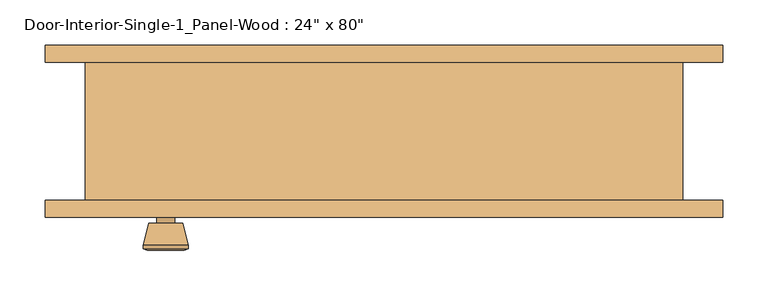
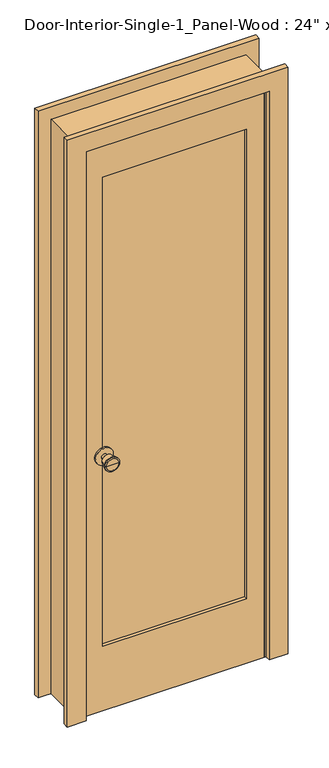
"""IFC4 building model written with IfcOpenShell, lengths in millimetres: door geometry."""

from ifc_helpers import new_model, si_unit, point, frame, frame_2d, origin, place, context, project, spatial, polyline, circle_curve, trimmed, segment, composite_curve, outline, extrude, faceted_brep, source, transform, mapped, element, save
from ifc_brep_helpers import plane_surface, cylinder_surface, revolved_surface, advanced_brep


def door_1d623f84(model_context):
    return source(origin(), model_context, "Body", "SolidModel", [
        advanced_brep(
        [(-241.3, -32.1, 914.4), (-251.3, -32.1, 914.4), (-231.3, -32.1, 914.4), (-220.8241324, 16.9, 914.4), (-261.7758676, 16.9, 914.4), (-241.3, 16.9, 914.4), (-216.3, 15.0721319, 914.4), (-266.3, 15.0721319, 914.4), (-216.3, 11.6084537, 914.4), (-266.3, 11.6084537, 914.4), (-222.663764, -13.1, 914.4), (-259.936236, -13.1, 914.4), (-231.3, -13.1, 914.4), (-251.3, -13.1, 914.4)],
        [
            (0, 1),
            (1, 2, circle_curve(frame((-241.3, -32.1, 914.4), z_axis=(0.0, -1.0, 0.0), x_axis=(-1.0, 0.0, 0.0)), 10.0)),
            (2, 0),
            (2, 1, circle_curve(frame((-241.3, -32.1, 914.4), z_axis=(0.0, -1.0, 0.0), x_axis=(-1.0, 0.0, 0.0)), 10.0)),
            (3, 4, circle_curve(frame((-241.3, 16.9, 914.4), z_axis=(0.0, 1.0, 0.0), x_axis=(-1.0, 0.0, 0.0)), 20.4758676)),
            (4, 5),
            (5, 3),
            (4, 3, circle_curve(frame((-241.3, 16.9, 914.4), z_axis=(0.0, 1.0, 0.0), x_axis=(-1.0, 0.0, 0.0)), 20.4758676)),
            (6, 7, circle_curve(frame((-241.3, 15.0721319, 914.4), z_axis=(0.0, 1.0, 0.0), x_axis=(-1.0, 0.0, 0.0)), 25.0)),
            (7, 4),
            (3, 6),
            (7, 6, circle_curve(frame((-241.3, 15.0721319, 914.4), z_axis=(0.0, 1.0, 0.0), x_axis=(-1.0, 0.0, 0.0)), 25.0)),
            (8, 9, circle_curve(frame((-241.3, 11.6084537, 914.4), z_axis=(0.0, 1.0, 0.0), x_axis=(-1.0, 0.0, 0.0)), 25.0)),
            (9, 7),
            (6, 8),
            (9, 8, circle_curve(frame((-241.3, 11.6084537, 914.4), z_axis=(0.0, 1.0, 0.0), x_axis=(-1.0, 0.0, 0.0)), 25.0)),
            (10, 11, circle_curve(frame((-241.3, -13.1, 914.4), z_axis=(0.0, 1.0, 0.0), x_axis=(-1.0, 0.0, 0.0)), 18.636236)),
            (11, 9),
            (8, 10),
            (11, 10, circle_curve(frame((-241.3, -13.1, 914.4), z_axis=(0.0, 1.0, 0.0), x_axis=(-1.0, 0.0, 0.0)), 18.636236)),
            (12, 13, circle_curve(frame((-241.3, -13.1, 914.4), z_axis=(0.0, 1.0, 0.0), x_axis=(-1.0, 0.0, 0.0)), 10.0)),
            (13, 11),
            (10, 12),
            (13, 12, circle_curve(frame((-241.3, -13.1, 914.4), z_axis=(0.0, 1.0, 0.0), x_axis=(-1.0, 0.0, 0.0)), 10.0)),
            (1, 13),
            (12, 2),
        ],
        [
            plane_surface(frame((-241.3, -32.1, 914.4), z_axis=(0.0, -1.0, 0.0), x_axis=(-1.0, 0.0, 0.0))),
            plane_surface(frame((-241.3, 16.9, 914.4), z_axis=(0.0, 1.0, 0.0), x_axis=(-1.0, 0.0, 0.0))),
            revolved_surface(polyline([(-261.7758676, 16.9, 914.4), (-266.3, 15.0721319, 914.4)]), (-241.3, -32.1, 914.4), (0.0, -1.0, 0.0)),
            cylinder_surface(frame((-241.3, -32.1, 914.4), z_axis=(0.0, -1.0, 0.0), x_axis=(-1.0, 0.0, 0.0)), 25.0),
            revolved_surface(polyline([(-266.3, 11.6084537, 914.4), (-259.936236, -13.1, 914.4)]), (-241.3, -32.1, 914.4), (0.0, -1.0, 0.0)),
            plane_surface(frame((-241.3, -13.1, 914.4), z_axis=(0.0, -1.0, 0.0), x_axis=(-1.0, 0.0, 0.0))),
            cylinder_surface(frame((-241.3, -32.1, 914.4), z_axis=(0.0, -1.0, 0.0), x_axis=(-1.0, 0.0, 0.0)), 10.0),
        ],
        [
            (0, [[1, 2, 3]]),
            (0, [[-3, 4, -1]]),
            (1, [[5, 6, 7]]),
            (1, [[8, -7, -6]]),
            (2, [[9, 10, -5, 11]]),
            (2, [[12, -11, -8, -10]]),
            (3, [[13, 14, -9, 15]]),
            (3, [[16, -15, -12, -14]]),
            (4, [[17, 18, -13, 19]]),
            (4, [[20, -19, -16, -18]]),
            (5, [[21, 22, -17, 23]]),
            (5, [[24, -23, -20, -22]]),
            (6, [[-2, 25, -21, 26]]),
            (6, [[-4, -26, -24, -25]]),
        ],
    ),
        extrude(outline(composite_curve([segment(trimmed(circle_curve(frame_2d((914.4, -241.3)), 30.0), [point((914.4, -271.3))], [point((914.4, -211.3))], False, "CARTESIAN"), True, "CONTINUOUS"), segment(trimmed(circle_curve(frame_2d((914.4, -241.3)), 30.0), [point((914.4, -211.3))], [point((914.4, -271.3))], False, "CARTESIAN"), True, "CONTINUOUS")], self_intersect=False)), frame((0.0, -38.1, 0.0), z_axis=(0.0, 1.0, 0.0), x_axis=(0.0, 0.0, 1.0)), (0.0, 0.0, 1.0), 6.0),
        advanced_brep(
        [(-241.3, -79.025, 914.4), (-231.3, -79.025, 914.4), (-251.3, -79.025, 914.4), (-220.8241324, -128.025, 914.4), (-241.3, -128.025, 914.4), (-261.7758676, -128.025, 914.4), (-216.3, -126.1971319, 914.4), (-266.3, -126.1971319, 914.4), (-216.3, -122.7334537, 914.4), (-266.3, -122.7334537, 914.4), (-222.663764, -98.025, 914.4), (-259.936236, -98.025, 914.4), (-231.3, -98.025, 914.4), (-251.3, -98.025, 914.4)],
        [
            (0, 1),
            (1, 2, circle_curve(frame((-241.3, -79.025, 914.4), z_axis=(0.0, 1.0, 0.0), x_axis=(-1.0, 0.0, 0.0)), 10.0)),
            (2, 0),
            (2, 1, circle_curve(frame((-241.3, -79.025, 914.4), z_axis=(0.0, 1.0, 0.0), x_axis=(-1.0, 0.0, 0.0)), 10.0)),
            (3, 4),
            (4, 5),
            (5, 3, circle_curve(frame((-241.3, -128.025, 914.4), z_axis=(0.0, -1.0, 0.0), x_axis=(-1.0, 0.0, 0.0)), 20.4758676)),
            (3, 5, circle_curve(frame((-241.3, -128.025, 914.4), z_axis=(0.0, -1.0, 0.0), x_axis=(-1.0, 0.0, 0.0)), 20.4758676)),
            (6, 3),
            (5, 7),
            (7, 6, circle_curve(frame((-241.3, -126.1971319, 914.4), z_axis=(0.0, -1.0, 0.0), x_axis=(-1.0, 0.0, 0.0)), 25.0)),
            (6, 7, circle_curve(frame((-241.3, -126.1971319, 914.4), z_axis=(0.0, -1.0, 0.0), x_axis=(-1.0, 0.0, 0.0)), 25.0)),
            (8, 6),
            (7, 9),
            (9, 8, circle_curve(frame((-241.3, -122.7334537, 914.4), z_axis=(0.0, -1.0, 0.0), x_axis=(-1.0, 0.0, 0.0)), 25.0)),
            (8, 9, circle_curve(frame((-241.3, -122.7334537, 914.4), z_axis=(0.0, -1.0, 0.0), x_axis=(-1.0, 0.0, 0.0)), 25.0)),
            (10, 8),
            (9, 11),
            (11, 10, circle_curve(frame((-241.3, -98.025, 914.4), z_axis=(0.0, -1.0, 0.0), x_axis=(-1.0, 0.0, 0.0)), 18.636236)),
            (10, 11, circle_curve(frame((-241.3, -98.025, 914.4), z_axis=(0.0, -1.0, 0.0), x_axis=(-1.0, 0.0, 0.0)), 18.636236)),
            (12, 10),
            (11, 13),
            (13, 12, circle_curve(frame((-241.3, -98.025, 914.4), z_axis=(0.0, -1.0, 0.0), x_axis=(-1.0, 0.0, 0.0)), 10.0)),
            (12, 13, circle_curve(frame((-241.3, -98.025, 914.4), z_axis=(0.0, -1.0, 0.0), x_axis=(-1.0, 0.0, 0.0)), 10.0)),
            (1, 12),
            (13, 2),
        ],
        [
            plane_surface(frame((-241.3, -79.025, 914.4), z_axis=(0.0, 1.0, 0.0), x_axis=(-1.0, 0.0, 0.0))),
            plane_surface(frame((-241.3, -128.025, 914.4), z_axis=(0.0, -1.0, 0.0), x_axis=(-1.0, 0.0, 0.0))),
            revolved_surface(polyline([(-261.7758676, -128.025, 914.4), (-266.3, -126.1971319, 914.4)]), (-241.3, -79.025, 914.4), (0.0, 1.0, 0.0)),
            cylinder_surface(frame((-241.3, -79.025, 914.4), z_axis=(0.0, 1.0, 0.0), x_axis=(-1.0, 0.0, 0.0)), 25.0),
            revolved_surface(polyline([(-266.3, -122.7334537, 914.4), (-259.936236, -98.025, 914.4)]), (-241.3, -79.025, 914.4), (0.0, 1.0, 0.0)),
            plane_surface(frame((-241.3, -98.025, 914.4), z_axis=(0.0, 1.0, 0.0), x_axis=(-1.0, 0.0, 0.0))),
            cylinder_surface(frame((-241.3, -79.025, 914.4), z_axis=(0.0, 1.0, 0.0), x_axis=(-1.0, 0.0, 0.0)), 10.0),
        ],
        [
            (0, [[1, 2, 3]]),
            (0, [[-3, 4, -1]]),
            (1, [[5, 6, 7]]),
            (1, [[-6, -5, 8]]),
            (2, [[9, -7, 10, 11]]),
            (2, [[-10, -8, -9, 12]]),
            (3, [[13, -11, 14, 15]]),
            (3, [[-14, -12, -13, 16]]),
            (4, [[17, -15, 18, 19]]),
            (4, [[-18, -16, -17, 20]]),
            (5, [[21, -19, 22, 23]]),
            (5, [[-22, -20, -21, 24]]),
            (6, [[25, -23, 26, -2]]),
            (6, [[-26, -24, -25, -4]]),
        ],
    ),
        extrude(outline(composite_curve([segment(trimmed(circle_curve(frame_2d((914.4, -241.3)), 30.0), [point((914.4, -271.3))], [point((914.4, -211.3))], False, "CARTESIAN"), True, "CONTINUOUS"), segment(trimmed(circle_curve(frame_2d((914.4, -241.3)), 30.0), [point((914.4, -211.3))], [point((914.4, -271.3))], False, "CARTESIAN"), True, "CONTINUOUS")], self_intersect=False)), frame((0.0, -79.025, 0.0), z_axis=(0.0, 1.0, 0.0), x_axis=(0.0, 0.0, 1.0)), (0.0, 0.0, 1.0), 6.0),
        extrude(outline(polyline([(244.475, -49.7416667), (244.475, -61.3833333), (-244.475, -61.3833333), (-244.475, -49.7416667), (244.475, -49.7416667)])), frame((0.0, 0.0, 231.775), z_axis=(0.0, 0.0, 1.0), x_axis=(1.0, 0.0, 0.0)), (0.0, 0.0, 1.0), 1681.1625),
        extrude(outline(polyline([(2032.0, -304.8), (0.0, -304.8), (0.0, 304.8), (2032.0, 304.8), (2032.0, -304.8)]), holes=[polyline([(1912.9375, -244.475), (1912.9375, 244.475), (231.775, 244.475), (231.775, -244.475), (1912.9375, -244.475)])]), frame((0.0, -73.025, 0.0), z_axis=(0.0, 1.0, 0.0), x_axis=(0.0, 0.0, 1.0)), (0.0, 0.0, 1.0), 34.925),
        faceted_brep([(330.2, -73.025, 0.0), (304.8, -73.025, 0.0), (304.8, -38.1, 0.0), (292.1, -38.1, 0.0), (292.1, -3.175, 0.0), (304.8, -3.175, 0.0), (304.8, 79.375, 0.0), (330.2, 79.375, 0.0), (330.2, 79.375, 2057.4), (330.2, -73.025, 2057.4), (304.8, 79.375, 2032.0), (-304.8, 79.375, 2032.0), (-304.8, 79.375, 0.0), (-330.2, 79.375, 0.0), (-330.2, 79.375, 2057.4), (304.8, -3.175, 2032.0), (292.1, -3.175, 2019.3), (-292.1, -3.175, 2019.3), (-292.1, -3.175, 0.0), (-304.8, -3.175, 0.0), (-304.8, -3.175, 2032.0), (292.1, -38.1, 2019.3), (304.8, -38.1, 2032.0), (-304.8, -38.1, 2032.0), (-304.8, -38.1, 0.0), (-292.1, -38.1, 0.0), (-292.1, -38.1, 2019.3), (304.8, -73.025, 2032.0), (-330.2, -73.025, 2057.4), (-330.2, -73.025, 0.0), (-304.8, -73.025, 0.0), (-304.8, -73.025, 2032.0)], [[[0, 1, 2, 3, 4, 5, 6, 7]], [[7, 8, 9, 0]], [[6, 10, 11, 12, 13, 14, 8, 7]], [[5, 15, 10, 6]], [[4, 16, 17, 18, 19, 20, 15, 5]], [[3, 21, 16, 4]], [[2, 22, 23, 24, 25, 26, 21, 3]], [[1, 27, 22, 2]], [[0, 9, 28, 29, 30, 31, 27, 1]], [[8, 14, 28, 9]], [[15, 20, 11, 10]], [[21, 26, 17, 16]], [[27, 31, 23, 22]], [[29, 13, 12, 19, 18, 25, 24, 30]], [[14, 13, 29, 28]], [[20, 19, 12, 11]], [[26, 25, 18, 17]], [[31, 30, 24, 23]]]),
        extrude(outline(polyline([(0.0, 374.65), (2101.85, 374.65), (2101.85, -374.65), (0.0, -374.65), (0.0, -311.15), (2038.35, -311.15), (2038.35, 311.15), (0.0, 311.15), (0.0, 374.65)])), frame((0.0, 79.375, 0.0), z_axis=(0.0, 1.0, 0.0), x_axis=(0.0, 0.0, 1.0)), (0.0, 0.0, 1.0), 19.05),
        extrude(outline(polyline([(0.0, 374.65), (2101.85, 374.65), (2101.85, -374.65), (0.0, -374.65), (0.0, -311.15), (2038.35, -311.15), (2038.35, 311.15), (0.0, 311.15), (0.0, 374.65)])), frame((0.0, -92.075, 0.0), z_axis=(0.0, 1.0, 0.0), x_axis=(0.0, 0.0, 1.0)), (0.0, 0.0, 1.0), 19.05),
    ])


if __name__ == "__main__":
    model = new_model("IFC4")
    model_context = context("Model", 3, world=origin())
    ifc_project = project(units=[si_unit("LENGTHUNIT", "METRE", prefix="MILLI")], contexts=[model_context])
    site = spatial("IfcSite", under=ifc_project)
    building = spatial("IfcBuilding", under=site)
    placement = place(None, origin())
    door_shape = door_1d623f84(model_context)
    element("IfcDoor", 1, ObjectType="Door-Interior-Single-1_Panel-Wood : 24\" x 80\"", at=placement, inside=building, context=model_context, shape_type="MappedRepresentation", body=[
        mapped(door_shape, transform((0.0, 0.0, 0.0), x_axis=(1.0, 0.0, 0.0), y_axis=(0.0, 1.0, 0.0), z_axis=(0.0, 0.0, 1.0))),
    ])
    save(model, "model.ifc")

# Revit data of these elements
# Type "Door-Interior-Single-1_Panel-Wood : 24\" x 80\""
#   Type Mark = "12"
#   Assembly Code = "C1020300"
#   Analytic Construction = "Wooden"
#   Top Rail = 0' - 4 11/16"
#   Thickness = 0' - 1 3/8"
#   Thermal Resistance (R) = 2.5876 (h·ft²·°F)/BTU
#   Swing Angle [instance default] = 90.00°
#   Stiles = 0' - 2 3/8"
#   Rough Width = 2' - 2"
#   Rough Height = 6' - 9"
#   Height = 6' - 8"
#   Width = 2' - 0"
#   Heat Transfer Coefficient (U) = 0.3865 BTU/(h·ft²·°F)
#   Bottom Rail = 0' - 9 1/8"
#   Trim Material = Cherry
#   Panel Material = Cherry
#   Frame Material = Cherry
#   Door Handle Material = Aluminum
#   Visual Light Transmittance = 0
#   Solar Heat Gain Coefficient = 0
#   Wall Closure = (empty or 0)
#   Function = (empty or 0)
# Element 1 (IfcDoor, "Door-Interior-Single-1_Panel-Wood : 24\" x 80\"")
#   Materials on its faces: "Cherry", "Aluminum"
# Materials
#   "Cherry": class "Wood", colour RGB 226 177 128, transparency 0, Description = "Prunus Serotina", Cost = 0
#   "Aluminum": class "Metal", colour RGB 247 247 247, transparency 0, Description = "Aluminum 6061", Cost = 0
